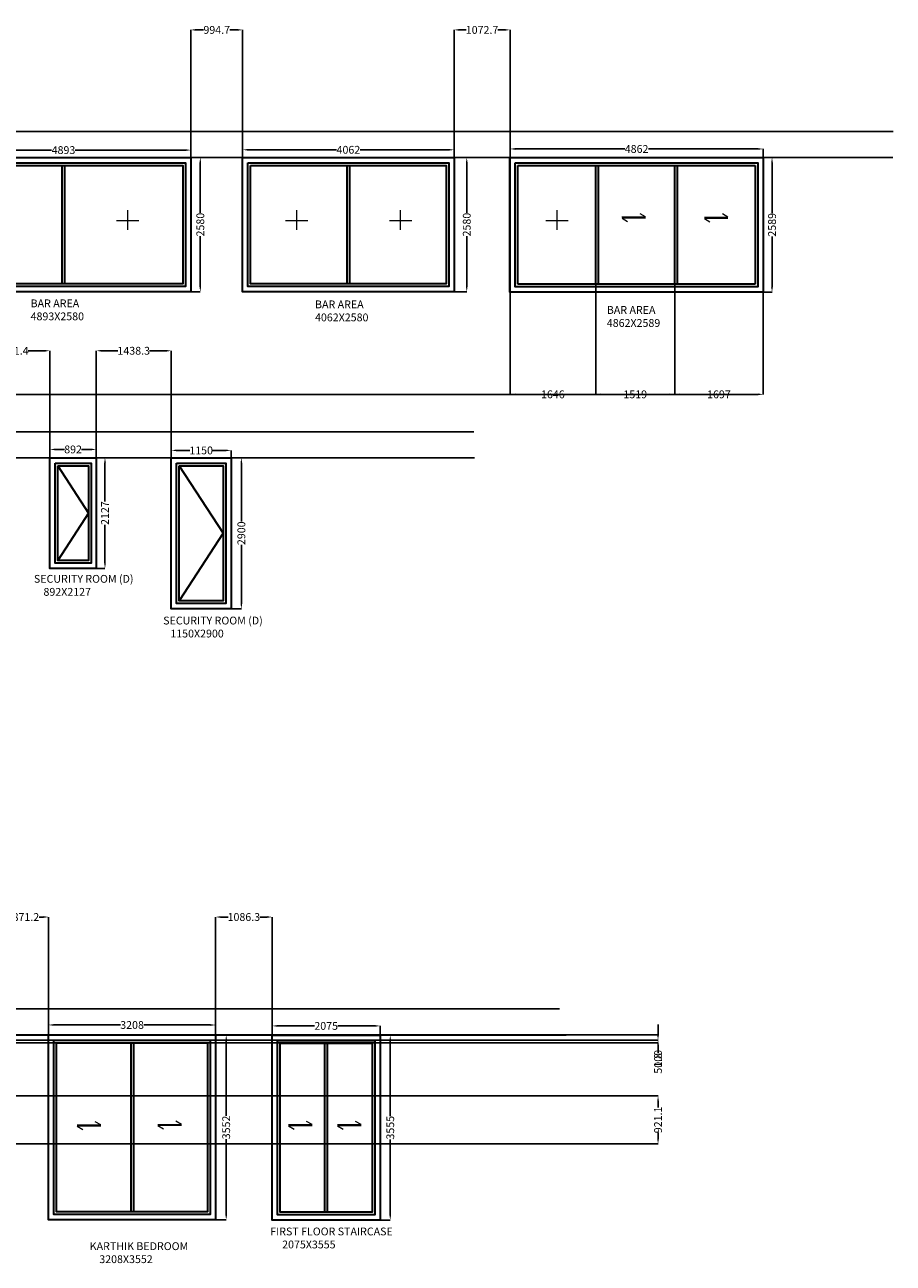
# Model space of a CAD drawing. Units: millimetres. Extents: x 16338 to 57165, y -4429 to 26237.
# Tile 6 of 6: x 40486 to 57165, y 2450 to 26237. Entities that reach past the tile are written whole.
import ezdxf

# ---------------------------------------------------------------- set-up
doc = ezdxf.new("R2010")
doc.units = ezdxf.units.MM
doc.header["$MEASUREMENT"] = 0
for name, color, linetype, lineweight in [('A-ANNO-DIMS', 5, 'Continuous', 18), ('A-ANNO-SYMB', 4, 'Continuous', 18), ('A-ANNO-TEXT', 3, 'Continuous', 18), ('A-ELEV', 8, 'Continuous', 25), ('A-GLAZ', 7, 'Continuous', 35)]:
    doc.layers.add(name, color=color, linetype=linetype, lineweight=lineweight)
doc.styles.get("Standard").update_dxf_attribs({"font": 'arial.ttf'})
doc.dimstyles.get("Standard").update_dxf_attribs({"dimtxt": 150, "dimasz": 100, "dimexe": 0.18, "dimexo": 0.0625, "dimgap": 0.09, "dimtad": 0, "dimdec": 0, "dimzin": 0, "dimdsep": 46, "dimtxsty": 'Standard', "dimcen": 0.09, "dimadec": 0, "dimazin": 0, "dimtfac": 1, "dimtdec": 0, "dimtofl": 0, "dimtmove": 0, "dimatfit": 3, "dimfxl": 1, "dimtolj": 1, "dimtzin": 0, "dimarcsym": 0})

# ---------------------------------------------------------------- blocks, each defined once
blk = doc.blocks.new('*D14')
at = {"layer": 'A-ANNO-DIMS', "color": 0, "lineweight": -2, "transparency": 16777216}
for p, q in [((38782, 23689), (38782, 23831)), ((38882, 23830), (41002, 23830)), ((43575, 23830), (41456, 23830)), ((43675, 23689), (43675, 23831))]:
    blk.add_line(p, q, dxfattribs=at)
at = {"layer": 'A-ANNO-DIMS', "color": 0, "transparency": 16777216}
for points in [[(38882, 23847), (38882, 23814), (38782, 23830)], [(43575, 23847), (43575, 23814), (43675, 23830)]]:
    blk.add_solid(points, dxfattribs=at)
at = {"layer": 'Defpoints', "color": 0, "transparency": 16777216}
for p in [(43675, 23830), (38782, 23689), (43675, 23689)]:
    blk.add_point(p, dxfattribs=at)
at = {"layer": 'A-ANNO-DIMS', "color": 0, "transparency": 16777216, "insert": (41229, 23830), "char_height": 150, "attachment_point": 5}
blk.add_mtext('\\A1;4893', dxfattribs=at)
blk = doc.blocks.new('*D15')
at = {"layer": 'A-ANNO-DIMS', "color": 0, "lineweight": -2, "transparency": 16777216}
for p, q in [((43675, 23689), (43857, 23689)), ((43857, 23589), (43857, 22624)), ((43857, 21209), (43857, 22174)), ((43675, 21109), (43857, 21109))]:
    blk.add_line(p, q, dxfattribs=at)
at = {"layer": 'A-ANNO-DIMS', "color": 0, "transparency": 16777216}
for points in [[(43840, 23589), (43873, 23589), (43857, 23689)], [(43840, 21209), (43873, 21209), (43857, 21109)]]:
    blk.add_solid(points, dxfattribs=at)
at = {"layer": 'Defpoints', "color": 0, "transparency": 16777216}
for p in [(43675, 23689), (43675, 21109), (43857, 21109)]:
    blk.add_point(p, dxfattribs=at)
at = {"layer": 'A-ANNO-DIMS', "color": 0, "transparency": 16777216, "insert": (43857, 22399), "char_height": 150, "attachment_point": 5, "rotation": 90}
blk.add_mtext('\\A1;2580', dxfattribs=at)
blk = doc.blocks.new('*D16')
at = {"layer": 'A-ANNO-DIMS', "color": 0, "lineweight": -2, "transparency": 16777216}
for p, q in [((44670, 23689), (44670, 23837)), ((44770, 23836), (46474, 23836)), ((48632, 23836), (46927, 23836)), ((48732, 23689), (48732, 23837))]:
    blk.add_line(p, q, dxfattribs=at)
at = {"layer": 'A-ANNO-DIMS', "color": 0, "transparency": 16777216}
for points in [[(44770, 23853), (44770, 23820), (44670, 23836)], [(48632, 23853), (48632, 23820), (48732, 23836)]]:
    blk.add_solid(points, dxfattribs=at)
at = {"layer": 'Defpoints', "color": 0, "transparency": 16777216}
for p in [(48732, 23836), (44670, 23689), (48732, 23689)]:
    blk.add_point(p, dxfattribs=at)
at = {"layer": 'A-ANNO-DIMS', "color": 0, "transparency": 16777216, "insert": (46701, 23836), "char_height": 150, "attachment_point": 5}
blk.add_mtext('\\A1;4062', dxfattribs=at)
blk = doc.blocks.new('*D17')
at = {"layer": 'A-ANNO-DIMS', "color": 0, "lineweight": -2, "transparency": 16777216}
for p, q in [((48732, 23689), (48974, 23689)), ((48974, 23589), (48974, 22624)), ((48974, 21209), (48974, 22174)), ((48732, 21109), (48974, 21109))]:
    blk.add_line(p, q, dxfattribs=at)
at = {"layer": 'A-ANNO-DIMS', "color": 0, "transparency": 16777216}
for points in [[(48957, 23589), (48990, 23589), (48974, 23689)], [(48957, 21209), (48990, 21209), (48974, 21109)]]:
    blk.add_solid(points, dxfattribs=at)
at = {"layer": 'Defpoints', "color": 0, "transparency": 16777216}
for p in [(48732, 23689), (48732, 21109), (48974, 21109)]:
    blk.add_point(p, dxfattribs=at)
at = {"layer": 'A-ANNO-DIMS', "color": 0, "transparency": 16777216, "insert": (48974, 22399), "char_height": 150, "attachment_point": 5, "rotation": 90}
blk.add_mtext('\\A1;2580', dxfattribs=at)
blk = doc.blocks.new('*D18')
at = {"layer": 'A-ANNO-DIMS', "color": 0, "lineweight": -2, "transparency": 16777216}
for p, q in [((49805, 23689), (49805, 23852)), ((49905, 23852), (52009, 23852)), ((54567, 23852), (52462, 23852)), ((54667, 23689), (54667, 23852))]:
    blk.add_line(p, q, dxfattribs=at)
at = {"layer": 'A-ANNO-DIMS', "color": 0, "transparency": 16777216}
for points in [[(49905, 23869), (49905, 23835), (49805, 23852)], [(54567, 23869), (54567, 23835), (54667, 23852)]]:
    blk.add_solid(points, dxfattribs=at)
at = {"layer": 'Defpoints', "color": 0, "transparency": 16777216}
for p in [(54667, 23852), (49805, 23689), (54667, 23689)]:
    blk.add_point(p, dxfattribs=at)
at = {"layer": 'A-ANNO-DIMS', "color": 0, "transparency": 16777216, "insert": (52236, 23852), "char_height": 150, "attachment_point": 5}
blk.add_mtext('\\A1;4862', dxfattribs=at)
blk = doc.blocks.new('*D19')
at = {"layer": 'A-ANNO-DIMS', "color": 0, "lineweight": -2, "transparency": 16777216}
for p, q in [((54667, 23689), (54837, 23689)), ((54837, 23589), (54837, 22620)), ((54837, 21200), (54837, 22169)), ((54667, 21100), (54837, 21100))]:
    blk.add_line(p, q, dxfattribs=at)
at = {"layer": 'A-ANNO-DIMS', "color": 0, "transparency": 16777216}
for points in [[(54820, 23589), (54854, 23589), (54837, 23689)], [(54820, 21200), (54854, 21200), (54837, 21100)]]:
    blk.add_solid(points, dxfattribs=at)
at = {"layer": 'Defpoints', "color": 0, "transparency": 16777216}
for p in [(54667, 23689), (54667, 21100), (54837, 21100)]:
    blk.add_point(p, dxfattribs=at)
at = {"layer": 'A-ANNO-DIMS', "color": 0, "transparency": 16777216, "insert": (54837, 22395), "char_height": 150, "attachment_point": 5, "rotation": 90}
blk.add_mtext('\\A1;2589', dxfattribs=at)
blk = doc.blocks.new('*D36')
at = {"layer": 'A-ANNO-DIMS', "color": 0, "lineweight": -2, "transparency": 16777216}
for p, q in [((40967, 17921), (40967, 18081)), ((41067, 18081), (41248, 18081)), ((41759, 18081), (41578, 18081)), ((41859, 17921), (41859, 18081))]:
    blk.add_line(p, q, dxfattribs=at)
at = {"layer": 'A-ANNO-DIMS', "color": 0, "transparency": 16777216}
for points in [[(41067, 18097), (41067, 18064), (40967, 18081)], [(41759, 18097), (41759, 18064), (41859, 18081)]]:
    blk.add_solid(points, dxfattribs=at)
at = {"layer": 'Defpoints', "color": 0, "transparency": 16777216}
for p in [(41859, 18081), (40967, 17921), (41859, 17921)]:
    blk.add_point(p, dxfattribs=at)
at = {"layer": 'A-ANNO-DIMS', "color": 0, "transparency": 16777216, "insert": (41413, 18081), "char_height": 150, "attachment_point": 5}
blk.add_mtext('\\A1;892', dxfattribs=at)
blk = doc.blocks.new('*D37')
at = {"layer": 'A-ANNO-DIMS', "color": 0, "lineweight": -2, "transparency": 16777216}
for p, q in [((41859, 17921), (42026, 17921)), ((42026, 17821), (42026, 17083)), ((42026, 15894), (42026, 16632)), ((41859, 15794), (42026, 15794))]:
    blk.add_line(p, q, dxfattribs=at)
at = {"layer": 'A-ANNO-DIMS', "color": 0, "transparency": 16777216}
for points in [[(42010, 17821), (42043, 17821), (42026, 17921)], [(42010, 15894), (42043, 15894), (42026, 15794)]]:
    blk.add_solid(points, dxfattribs=at)
at = {"layer": 'Defpoints', "color": 0, "transparency": 16777216}
for p in [(41859, 17921), (41859, 15794), (42026, 15794)]:
    blk.add_point(p, dxfattribs=at)
at = {"layer": 'A-ANNO-DIMS', "color": 0, "transparency": 16777216, "insert": (42026, 16858), "char_height": 150, "attachment_point": 5, "rotation": 90}
blk.add_mtext('\\A1;2127', dxfattribs=at)
blk = doc.blocks.new('*D38')
at = {"layer": 'A-ANNO-DIMS', "color": 0, "lineweight": -2, "transparency": 16777216}
for p, q in [((43298, 17921), (43298, 18062)), ((43398, 18062), (43656, 18062)), ((44348, 18062), (44089, 18062)), ((44448, 17921), (44448, 18062))]:
    blk.add_line(p, q, dxfattribs=at)
at = {"layer": 'A-ANNO-DIMS', "color": 0, "transparency": 16777216}
for points in [[(43398, 18079), (43398, 18046), (43298, 18062)], [(44348, 18079), (44348, 18046), (44448, 18062)]]:
    blk.add_solid(points, dxfattribs=at)
at = {"layer": 'Defpoints', "color": 0, "transparency": 16777216}
for p in [(43298, 17921), (44448, 18062), (44448, 17921)]:
    blk.add_point(p, dxfattribs=at)
at = {"layer": 'A-ANNO-DIMS', "color": 0, "transparency": 16777216, "insert": (43873, 18062), "char_height": 150, "attachment_point": 5}
blk.add_mtext('\\A1;1150', dxfattribs=at)
blk = doc.blocks.new('*D39')
at = {"layer": 'A-ANNO-DIMS', "color": 0, "lineweight": -2, "transparency": 16777216}
for p, q in [((44448, 17921), (44646, 17921)), ((44645, 17821), (44645, 16696)), ((44645, 15121), (44645, 16246)), ((44448, 15021), (44646, 15021))]:
    blk.add_line(p, q, dxfattribs=at)
at = {"layer": 'A-ANNO-DIMS', "color": 0, "transparency": 16777216}
for points in [[(44629, 17821), (44662, 17821), (44645, 17921)], [(44629, 15121), (44662, 15121), (44645, 15021)]]:
    blk.add_solid(points, dxfattribs=at)
at = {"layer": 'Defpoints', "color": 0, "transparency": 16777216}
for p in [(44448, 17921), (44448, 15021), (44645, 15021)]:
    blk.add_point(p, dxfattribs=at)
at = {"layer": 'A-ANNO-DIMS', "color": 0, "transparency": 16777216, "insert": (44645, 16471), "char_height": 150, "attachment_point": 5, "rotation": 90}
blk.add_mtext('\\A1;2900', dxfattribs=at)
blk = doc.blocks.new('*D67')
at = {"layer": 'A-ANNO-DIMS', "color": 0, "lineweight": -2, "transparency": 16777216}
for p, q in [((40942, 6834), (40942, 7026)), ((41042, 7026), (42322, 7026)), ((44050, 7026), (42770, 7026)), ((44150, 6834), (44150, 7026))]:
    blk.add_line(p, q, dxfattribs=at)
at = {"layer": 'A-ANNO-DIMS', "color": 0, "transparency": 16777216}
for points in [[(41042, 7043), (41042, 7009), (40942, 7026)], [(44050, 7043), (44050, 7009), (44150, 7026)]]:
    blk.add_solid(points, dxfattribs=at)
at = {"layer": 'Defpoints', "color": 0, "transparency": 16777216}
for p in [(44150, 7026), (40942, 6834), (44150, 6834)]:
    blk.add_point(p, dxfattribs=at)
at = {"layer": 'A-ANNO-DIMS', "color": 0, "transparency": 16777216, "insert": (42546, 7026), "char_height": 150, "attachment_point": 5}
blk.add_mtext('\\A1;3208', dxfattribs=at)
blk = doc.blocks.new('*D68')
at = {"layer": 'A-ANNO-DIMS', "color": 0, "lineweight": -2, "transparency": 16777216}
for p, q in [((44150, 6834), (44355, 6834)), ((44354, 6734), (44354, 5281)), ((44354, 3382), (44354, 4835)), ((44150, 3282), (44355, 3282))]:
    blk.add_line(p, q, dxfattribs=at)
at = {"layer": 'A-ANNO-DIMS', "color": 0, "transparency": 16777216}
for points in [[(44338, 6734), (44371, 6734), (44354, 6834)], [(44338, 3382), (44371, 3382), (44354, 3282)]]:
    blk.add_solid(points, dxfattribs=at)
at = {"layer": 'Defpoints', "color": 0, "transparency": 16777216}
for p in [(44150, 6834), (44150, 3282), (44354, 3282)]:
    blk.add_point(p, dxfattribs=at)
at = {"layer": 'A-ANNO-DIMS', "color": 0, "transparency": 16777216, "insert": (44354, 5058), "char_height": 150, "attachment_point": 5, "rotation": 90}
blk.add_mtext('\\A1;3552', dxfattribs=at)
blk = doc.blocks.new('*D69')
at = {"layer": 'A-ANNO-DIMS', "color": 0, "lineweight": -2, "transparency": 16777216}
for p, q in [((45236, 6830), (45236, 7008)), ((45336, 7008), (46048, 7008)), ((47211, 7008), (46500, 7008)), ((47311, 6830), (47311, 7008))]:
    blk.add_line(p, q, dxfattribs=at)
at = {"layer": 'A-ANNO-DIMS', "color": 0, "transparency": 16777216}
for points in [[(45336, 7025), (45336, 6992), (45236, 7008)], [(47211, 7025), (47211, 6992), (47311, 7008)]]:
    blk.add_solid(points, dxfattribs=at)
at = {"layer": 'Defpoints', "color": 0, "transparency": 16777216}
for p in [(47311, 7008), (45236, 6830), (47311, 6830)]:
    blk.add_point(p, dxfattribs=at)
at = {"layer": 'A-ANNO-DIMS', "color": 0, "transparency": 16777216, "insert": (46274, 7008), "char_height": 150, "attachment_point": 5}
blk.add_mtext('\\A1;2075', dxfattribs=at)
blk = doc.blocks.new('*D70')
at = {"layer": 'A-ANNO-DIMS', "color": 0, "lineweight": -2, "transparency": 16777216}
for p, q in [((47311, 6830), (47505, 6830)), ((47505, 6730), (47505, 5277)), ((47505, 3375), (47505, 4828)), ((47311, 3275), (47505, 3275))]:
    blk.add_line(p, q, dxfattribs=at)
at = {"layer": 'A-ANNO-DIMS', "color": 0, "transparency": 16777216}
for points in [[(47488, 6730), (47521, 6730), (47505, 6830)], [(47488, 3375), (47521, 3375), (47505, 3275)]]:
    blk.add_solid(points, dxfattribs=at)
at = {"layer": 'Defpoints', "color": 0, "transparency": 16777216}
for p in [(47311, 6830), (47311, 3275), (47505, 3275)]:
    blk.add_point(p, dxfattribs=at)
at = {"layer": 'A-ANNO-DIMS', "color": 0, "transparency": 16777216, "insert": (47505, 5053), "char_height": 150, "attachment_point": 5, "rotation": 90}
blk.add_mtext('\\A1;3555', dxfattribs=at)
blk = doc.blocks.new('SLIDE-ARROW-L')
for p, q in [((454, 0), (347, 62)), ((0, 0), (454, 0))]:
    blk.add_line(p, q)
blk = doc.blocks.new('*D89')
at = {"layer": 'A-ANNO-DIMS', "color": 0, "lineweight": -2, "transparency": 16777216}
for p, q in [((43675, 23689), (43675, 26139)), ((43775, 26139), (43919, 26139)), ((44570, 26139), (44426, 26139)), ((44670, 23689), (44670, 26139))]:
    blk.add_line(p, q, dxfattribs=at)
at = {"layer": 'A-ANNO-DIMS', "color": 0, "transparency": 16777216}
for points in [[(43775, 26156), (43775, 26122), (43675, 26139)], [(44570, 26156), (44570, 26122), (44670, 26139)]]:
    blk.add_solid(points, dxfattribs=at)
at = {"layer": 'Defpoints', "color": 0, "transparency": 16777216}
for p in [(44670, 26139), (43675, 23689), (44670, 23689)]:
    blk.add_point(p, dxfattribs=at)
at = {"layer": 'A-ANNO-DIMS', "color": 0, "transparency": 16777216, "insert": (44172, 26139), "char_height": 150, "attachment_point": 5}
blk.add_mtext('\\A1;994.7', dxfattribs=at)
blk = doc.blocks.new('*D90')
at = {"layer": 'A-ANNO-DIMS', "color": 0, "lineweight": -2, "transparency": 16777216}
for p, q in [((48732, 23689), (48732, 26139)), ((48832, 26139), (48964, 26139)), ((49705, 26139), (49573, 26139)), ((49805, 23689), (49805, 26139))]:
    blk.add_line(p, q, dxfattribs=at)
at = {"layer": 'A-ANNO-DIMS', "color": 0, "transparency": 16777216}
for points in [[(48832, 26156), (48832, 26122), (48732, 26139)], [(49705, 26156), (49705, 26122), (49805, 26139)]]:
    blk.add_solid(points, dxfattribs=at)
at = {"layer": 'Defpoints', "color": 0, "transparency": 16777216}
for p in [(49805, 26139), (48732, 23689), (49805, 23689)]:
    blk.add_point(p, dxfattribs=at)
at = {"layer": 'A-ANNO-DIMS', "color": 0, "transparency": 16777216, "insert": (49268, 26139), "char_height": 150, "attachment_point": 5}
blk.add_mtext('\\A1;1072.7', dxfattribs=at)
blk = doc.blocks.new('*D91')
at = {"layer": 'A-ANNO-DIMS', "color": 0, "lineweight": -2, "transparency": 16777216}
for p, q in [((19179, 21089), (19179, 19139)), ((54667, 21100), (54667, 19139)), ((19279, 19139), (36641, 19139)), ((54567, 19139), (37205, 19139))]:
    blk.add_line(p, q, dxfattribs=at)
at = {"layer": 'A-ANNO-DIMS', "color": 0, "transparency": 16777216}
for points in [[(19279, 19156), (19279, 19122), (19179, 19139)], [(54567, 19156), (54567, 19122), (54667, 19139)]]:
    blk.add_solid(points, dxfattribs=at)
at = {"layer": 'Defpoints', "color": 0, "transparency": 16777216}
for p in [(19179, 21089), (54667, 21100), (54667, 19139)]:
    blk.add_point(p, dxfattribs=at)
at = {"layer": 'A-ANNO-DIMS', "color": 0, "transparency": 16777216, "insert": (36923, 19139), "char_height": 150, "attachment_point": 5}
blk.add_mtext('\\A1;35487', dxfattribs=at)
blk = doc.blocks.new('*D92')
at = {"layer": 'A-ANNO-DIMS', "color": 0, "lineweight": -2, "transparency": 16777216}
for p, q in [((49805, 23689), (49805, 19139)), ((51451, 23537), (51451, 19139)), ((49905, 19139), (50411, 19139)), ((51351, 19139), (50845, 19139))]:
    blk.add_line(p, q, dxfattribs=at)
at = {"layer": 'A-ANNO-DIMS', "color": 0, "transparency": 16777216}
for points in [[(49905, 19156), (49905, 19122), (49805, 19139)], [(51351, 19156), (51351, 19122), (51451, 19139)]]:
    blk.add_solid(points, dxfattribs=at)
at = {"layer": 'Defpoints', "color": 0, "transparency": 16777216}
for p in [(49805, 23689), (51451, 23537), (51451, 19139)]:
    blk.add_point(p, dxfattribs=at)
at = {"layer": 'A-ANNO-DIMS', "color": 0, "transparency": 16777216, "insert": (50628, 19139), "char_height": 150, "attachment_point": 5}
blk.add_mtext('\\A1;1646', dxfattribs=at)
blk = doc.blocks.new('*D93')
at = {"layer": 'A-ANNO-DIMS', "color": 0, "lineweight": -2, "transparency": 16777216}
for p, q in [((51451, 23537), (51451, 19139)), ((52970, 23537), (52970, 19139)), ((51551, 19139), (51993, 19139)), ((52870, 19139), (52427, 19139))]:
    blk.add_line(p, q, dxfattribs=at)
at = {"layer": 'A-ANNO-DIMS', "color": 0, "transparency": 16777216}
for points in [[(51551, 19156), (51551, 19122), (51451, 19139)], [(52870, 19156), (52870, 19122), (52970, 19139)]]:
    blk.add_solid(points, dxfattribs=at)
at = {"layer": 'Defpoints', "color": 0, "transparency": 16777216}
for p in [(51451, 23537), (52970, 23537), (52970, 19139)]:
    blk.add_point(p, dxfattribs=at)
at = {"layer": 'A-ANNO-DIMS', "color": 0, "transparency": 16777216, "insert": (52210, 19139), "char_height": 150, "attachment_point": 5}
blk.add_mtext('\\A1;1519', dxfattribs=at)
blk = doc.blocks.new('*D94')
at = {"layer": 'A-ANNO-DIMS', "color": 0, "lineweight": -2, "transparency": 16777216}
for p, q in [((54667, 23689), (54667, 19139)), ((52970, 23537), (52970, 19139)), ((53070, 19139), (53601, 19139)), ((54567, 19139), (54035, 19139))]:
    blk.add_line(p, q, dxfattribs=at)
at = {"layer": 'A-ANNO-DIMS', "color": 0, "transparency": 16777216}
for points in [[(53070, 19156), (53070, 19122), (52970, 19139)], [(54567, 19156), (54567, 19122), (54667, 19139)]]:
    blk.add_solid(points, dxfattribs=at)
at = {"layer": 'Defpoints', "color": 0, "transparency": 16777216}
for p in [(54667, 23689), (52970, 23537), (54667, 19139)]:
    blk.add_point(p, dxfattribs=at)
at = {"layer": 'A-ANNO-DIMS', "color": 0, "transparency": 16777216, "insert": (53818, 19139), "char_height": 150, "attachment_point": 5}
blk.add_mtext('\\A1;1697', dxfattribs=at)
blk = doc.blocks.new('*D102')
at = {"layer": 'A-ANNO-DIMS', "color": 0, "lineweight": -2, "transparency": 16777216}
for p, q in [((39526, 17921), (39526, 19976)), ((39626, 19976), (39943, 19976)), ((40867, 19976), (40551, 19976)), ((40967, 17921), (40967, 19976))]:
    blk.add_line(p, q, dxfattribs=at)
at = {"layer": 'A-ANNO-DIMS', "color": 0, "transparency": 16777216}
for points in [[(39626, 19993), (39626, 19959), (39526, 19976)], [(40867, 19993), (40867, 19959), (40967, 19976)]]:
    blk.add_solid(points, dxfattribs=at)
at = {"layer": 'Defpoints', "color": 0, "transparency": 16777216}
for p in [(40967, 19976), (39526, 17921), (40967, 17921)]:
    blk.add_point(p, dxfattribs=at)
at = {"layer": 'A-ANNO-DIMS', "color": 0, "transparency": 16777216, "insert": (40247, 19976), "char_height": 150, "attachment_point": 5}
blk.add_mtext('\\A1;1441.4', dxfattribs=at)
blk = doc.blocks.new('*D103')
at = {"layer": 'A-ANNO-DIMS', "color": 0, "lineweight": -2, "transparency": 16777216}
for p, q in [((41859, 17921), (41859, 19976)), ((41959, 19976), (42274, 19976)), ((43198, 19976), (42883, 19976)), ((43298, 17921), (43298, 19976))]:
    blk.add_line(p, q, dxfattribs=at)
at = {"layer": 'A-ANNO-DIMS', "color": 0, "transparency": 16777216}
for points in [[(41959, 19993), (41959, 19959), (41859, 19976)], [(43198, 19993), (43198, 19959), (43298, 19976)]]:
    blk.add_solid(points, dxfattribs=at)
at = {"layer": 'Defpoints', "color": 0, "transparency": 16777216}
for p in [(43298, 19976), (41859, 17921), (43298, 17921)]:
    blk.add_point(p, dxfattribs=at)
at = {"layer": 'A-ANNO-DIMS', "color": 0, "transparency": 16777216, "insert": (42578, 19976), "char_height": 150, "attachment_point": 5}
blk.add_mtext('\\A1;1438.3', dxfattribs=at)
blk = doc.blocks.new('*D116')
at = {"layer": 'A-ANNO-DIMS', "color": 0, "lineweight": -2, "transparency": 16777216}
for p, q in [((40071, 6835), (40071, 9100)), ((40171, 9100), (40254, 9100)), ((40842, 9100), (40759, 9100)), ((40942, 6834), (40942, 9100))]:
    blk.add_line(p, q, dxfattribs=at)
at = {"layer": 'A-ANNO-DIMS', "color": 0, "transparency": 16777216}
for points in [[(40171, 9117), (40171, 9083), (40071, 9100)], [(40842, 9117), (40842, 9083), (40942, 9100)]]:
    blk.add_solid(points, dxfattribs=at)
at = {"layer": 'Defpoints', "color": 0, "transparency": 16777216}
for p in [(40942, 9100), (40071, 6835), (40942, 6834)]:
    blk.add_point(p, dxfattribs=at)
at = {"layer": 'A-ANNO-DIMS', "color": 0, "transparency": 16777216, "insert": (40507, 9100), "char_height": 150, "attachment_point": 5}
blk.add_mtext('\\A1;871.2', dxfattribs=at)
blk = doc.blocks.new('*D117')
at = {"layer": 'A-ANNO-DIMS', "color": 0, "lineweight": -2, "transparency": 16777216}
for p, q in [((44150, 6834), (44150, 9100)), ((44250, 9100), (44389, 9100)), ((45136, 9100), (44998, 9100)), ((45236, 6830), (45236, 9100))]:
    blk.add_line(p, q, dxfattribs=at)
at = {"layer": 'A-ANNO-DIMS', "color": 0, "transparency": 16777216}
for points in [[(44250, 9117), (44250, 9083), (44150, 9100)], [(45136, 9117), (45136, 9083), (45236, 9100)]]:
    blk.add_solid(points, dxfattribs=at)
at = {"layer": 'Defpoints', "color": 0, "transparency": 16777216}
for p in [(45236, 9100), (44150, 6834), (45236, 6830)]:
    blk.add_point(p, dxfattribs=at)
at = {"layer": 'A-ANNO-DIMS', "color": 0, "transparency": 16777216, "insert": (44693, 9100), "char_height": 150, "attachment_point": 5}
blk.add_mtext('\\A1;1086.3', dxfattribs=at)
blk = doc.blocks.new('*D126')
at = {"layer": 'A-ANNO-DIMS', "color": 0, "lineweight": -2, "transparency": 16777216}
for p, q in [((52648, 6935), (52648, 7035)), ((23725, 6735), (52648, 6735)), ((23825, 6835), (52648, 6835)), ((52648, 6635), (52648, 6535))]:
    blk.add_line(p, q, dxfattribs=at)
at = {"layer": 'A-ANNO-DIMS', "color": 0, "transparency": 16777216}
for points in [[(52631, 6935), (52665, 6935), (52648, 6835)], [(52631, 6635), (52665, 6635), (52648, 6735)]]:
    blk.add_solid(points, dxfattribs=at)
at = {"layer": 'Defpoints', "color": 0, "transparency": 16777216}
for p in [(23725, 6735), (23825, 6835), (52648, 6735)]:
    blk.add_point(p, dxfattribs=at)
at = {"layer": 'A-ANNO-DIMS', "color": 0, "transparency": 16777216, "insert": (52648, 6377), "char_height": 150, "attachment_point": 5, "rotation": 90}
blk.add_mtext('\\A1;100', dxfattribs=at)
blk = doc.blocks.new('*D127')
at = {"layer": 'A-ANNO-DIMS', "color": 0, "lineweight": -2, "transparency": 16777216}
for p, q in [((52648, 6835), (52648, 6935)), ((23674, 6684), (52648, 6684)), ((23725, 6735), (52648, 6735)), ((52648, 6584), (52648, 6484))]:
    blk.add_line(p, q, dxfattribs=at)
at = {"layer": 'A-ANNO-DIMS', "color": 0, "transparency": 16777216}
for points in [[(52631, 6835), (52665, 6835), (52648, 6735)], [(52631, 6584), (52665, 6584), (52648, 6684)]]:
    blk.add_solid(points, dxfattribs=at)
at = {"layer": 'Defpoints', "color": 0, "transparency": 16777216}
for p in [(23674, 6684), (23725, 6735), (52648, 6684)]:
    blk.add_point(p, dxfattribs=at)
at = {"layer": 'A-ANNO-DIMS', "color": 0, "transparency": 16777216, "insert": (52648, 6289), "char_height": 150, "attachment_point": 5, "rotation": 90}
blk.add_mtext('\\A1;50.8', dxfattribs=at)
blk = doc.blocks.new('*D132')
at = {"layer": 'A-ANNO-DIMS', "color": 0, "lineweight": -2, "transparency": 16777216}
for p, q in [((23674, 5663), (52648, 5663)), ((52648, 5563), (52648, 5441)), ((52648, 4842), (52648, 4964)), ((23616, 4742), (52648, 4742))]:
    blk.add_line(p, q, dxfattribs=at)
at = {"layer": 'A-ANNO-DIMS', "color": 0, "transparency": 16777216}
for points in [[(52631, 5563), (52665, 5563), (52648, 5663)], [(52631, 4842), (52665, 4842), (52648, 4742)]]:
    blk.add_solid(points, dxfattribs=at)
at = {"layer": 'Defpoints', "color": 0, "transparency": 16777216}
for p in [(23674, 5663), (52648, 5663), (23616, 4742)]:
    blk.add_point(p, dxfattribs=at)
at = {"layer": 'A-ANNO-DIMS', "color": 0, "transparency": 16777216, "insert": (52648, 5203), "char_height": 150, "attachment_point": 5, "rotation": 90}
blk.add_mtext('\\A1;921.1', dxfattribs=at)

msp = doc.modelspace()

# ---------------------------------------------------------------- linework, layer by layer
at = {"layer": 'A-ANNO-DIMS'}
for p in [(51475.99, 21252.42), (52995.06, 21252.42)]:
    msp.add_point(p, dxfattribs=at)
at = {"layer": 'A-ANNO-SYMB'}
for p, q in [((42462.86, 22298.38), (42462.86, 22676.6)), ((45709.68, 22298.38), (45709.68, 22676.6)), ((47702.87, 22298.38), (47702.87, 22676.6)), ((50708.19, 22298.38), (50708.19, 22676.6)), ((42248.45, 22479.47), (42677.27, 22479.47)), ((45495.27, 22479.47), (45924.09, 22479.47)), ((47488.46, 22479.47), (47917.28, 22479.47)), ((50493.78, 22479.47), (50922.6, 22479.47))]:
    msp.add_line(p, q, dxfattribs=at)
at = {"layer": 'A-ELEV'}
for p, q in [((18334.8, 24189.02), (57164.77, 24189.02)), ((18334.8, 23689.02), (57154.46, 23689.02)), ((18334.8, 18421.15), (49111.23, 18421.15)), ((18334.8, 17921.15), (49122.07, 17921.15)), ((18209.23, 7335.1), (50757.08, 7335.1)), ((18201.83, 6834.85), (50882.91, 6829.39))]:
    msp.add_line(p, q, dxfattribs=at)
at = {"layer": 'A-GLAZ'}
for p, q in [((41203.19, 21261.42), (41203.19, 23536.62)), ((41253.99, 21261.42), (41253.99, 23536.62)), ((46675.42, 21261.42), (46675.42, 23536.62)), ((46726.22, 21261.42), (46726.22, 23536.62)), ((49956.93, 23536.62), (54514.13, 23536.62)), ((49956.93, 21252.42), (49956.93, 23536.62)), ((51450.59, 21252.42), (51450.59, 23536.62)), ((51501.39, 21252.42), (51501.39, 23536.62)), ((52969.66, 21252.42), (52969.66, 23536.62)), ((53020.46, 21252.42), (53020.46, 23536.62)), ((54514.13, 23536.62), (54514.13, 21252.42)), ((54514.13, 21252.42), (49956.93, 21252.42)), ((41119.74, 17768.75), (41706.94, 16857.65)), ((43450.06, 17768.75), (44295.26, 16471.15)), ((41706.94, 16857.65), (41119.74, 15946.55)), ((44295.26, 16471.15), (43450.06, 15173.55)), ((42520.74, 6681.8), (42520.74, 3434.6)), ((42571.54, 6681.8), (42571.54, 3434.6)), ((46248.52, 3427.73), (46248.52, 6677.93)), ((46299.32, 3427.73), (46299.32, 6677.93))]:
    msp.add_line(p, q, dxfattribs=at)
for points in [[(38782.09, 23689.02), (43675.09, 23689.02), (43675.09, 21109.02), (38782.09, 21109.02)], [(38883.69, 23587.42), (43573.49, 23587.42), (43573.49, 21210.62), (38883.69, 21210.62)], [(44669.82, 23689.02), (48731.82, 23689.02), (48731.82, 21109.02), (44669.82, 21109.02)], [(44771.42, 23587.42), (48630.22, 23587.42), (48630.22, 21210.62), (44771.42, 21210.62)], [(49804.53, 23689.02), (54666.53, 23689.02), (54666.53, 21100.02), (49804.53, 21100.02)], [(49906.13, 23587.42), (54564.93, 23587.42), (54564.93, 21201.62), (49906.13, 21201.62)], [(38934.49, 23536.62), (43522.69, 23536.62), (43522.69, 21261.42), (38934.49, 21261.42)], [(44822.22, 23536.62), (48579.42, 23536.62), (48579.42, 21261.42), (44822.22, 21261.42)], [(40967.34, 17921.15), (41859.34, 17921.15), (41859.34, 15794.15), (40967.34, 15794.15)], [(43297.66, 17921.15), (44447.66, 17921.15), (44447.66, 15021.15), (43297.66, 15021.15)], [(41068.94, 17819.55), (41757.74, 17819.55), (41757.74, 15895.75), (41068.94, 15895.75)], [(41119.74, 17768.75), (41706.94, 17768.75), (41706.94, 15946.55), (41119.74, 15946.55)], [(43399.26, 17819.55), (44346.06, 17819.55), (44346.06, 15122.75), (43399.26, 15122.75)], [(43450.06, 17768.75), (44295.26, 17768.75), (44295.26, 15173.55), (43450.06, 15173.55)], [(40942.14, 6834.2), (44150.14, 6834.2), (44150.14, 3282.2), (40942.14, 3282.2)], [(41043.74, 6732.6), (44048.54, 6732.6), (44048.54, 3383.8), (41043.74, 3383.8)], [(41094.54, 6681.8), (43997.74, 6681.8), (43997.74, 3434.6), (41094.54, 3434.6)], [(45236.42, 6830.33), (47311.42, 6830.33), (47311.42, 3275.33), (45236.42, 3275.33)], [(45338.02, 6728.73), (47209.82, 6728.73), (47209.82, 3376.93), (45338.02, 3376.93)], [(45388.82, 6677.93), (47159.02, 6677.93), (47159.02, 3427.73), (45388.82, 3427.73)]]:
    msp.add_lwpolyline(points, close=True, dxfattribs=at)

# ---------------------------------------------------------------- block references
at = {"layer": 'A-ANNO-SYMB'}
for p in [(51955.59, 22545.86), (53537.03, 22541.17), (41490.33, 5106.84), (43041.75, 5117.24), (45552.37, 5113.38), (46491.06, 5113.38)]:
    msp.add_blockref('SLIDE-ARROW-L', p, dxfattribs=at)
at = {"layer": 'A-ANNO-SYMB', "rotation": 180}
for p in [(52409.79, 22521.2), (53991.23, 22516.52), (41944.53, 5082.19), (43495.95, 5092.59), (46006.57, 5088.72), (46945.26, 5088.72)]:
    msp.add_blockref('SLIDE-ARROW-L', p, dxfattribs=at)

# ---------------------------------------------------------------- texts
at = {"layer": 'A-ANNO-TEXT', "char_height": 150, "attachment_point": 1}
for s, insert in [('BAR AREA\\P4893X2580', (40597.6, 20961.52)), ('BAR AREA\\P4062X2580', (46060.13, 20941.98)), ('BAR AREA\\P4862X2589', (51664.52, 20834.71)), ('SECURITY ROOM (D)\\P    892X2127', (40661.38, 15670.31)), ('SECURITY ROOM (D)\\P   1150X2900', (43143.97, 14869.2)), ('FIRST FLOOR STAIRCASE\\P     2075X3555', (45199.59, 3135.03)), ('\\PKARTHIK BEDROOM\\P    3208X3552', (41733.24, 3102.75))]:
    msp.add_mtext_dynamic_manual_height_columns(s, width=7094.9176, gutter_width=1, heights=[0], dxfattribs=dict(at, insert=insert))

# ---------------------------------------------------------------- dimensions: what is measured, and where the dimension line sits
at = {"layer": 'A-ANNO-DIMS'}
for base, p1, p2, override, picture, middle in [((44669.82, 26139.02), (43675.09, 23689.02), (44669.82, 23689.02), {"dimdec": 1, "dimlfac": 1, "dimrnd": 0, "dimzin": 0, "dimdsep": 46, "dimlunit": 2}, '*D89', (44172.45, 26139.02)), ((49804.53, 26139.02), (48731.82, 23689.02), (49804.53, 23689.02), {"dimdec": 1, "dimlfac": 1, "dimrnd": 0, "dimzin": 0, "dimdsep": 46, "dimlunit": 2}, '*D90', (49268.17, 26139.02)), ((43675.09, 23830.45), (38782.09, 23689.02), (43675.09, 23689.02), {"dimclrd": 0, "dimclre": 0, "dimclrt": 0}, '*D14', (41228.59, 23830.45)), ((48731.82, 23836.37), (44669.82, 23689.02), (48731.82, 23689.02), {"dimclrd": 0, "dimclre": 0, "dimclrt": 0}, '*D16', (46700.82, 23836.37)), ((54666.53, 23851.85), (49804.53, 23689.02), (54666.53, 23689.02), {"dimclrd": 0, "dimclre": 0, "dimclrt": 0}, '*D18', (52235.53, 23851.85)), ((51450.59, 19139.02), (49804.53, 23689.02), (51450.59, 23536.62), {"dimdec": 0, "dimlfac": 1, "dimrnd": 0, "dimzin": 0, "dimdsep": 46, "dimlunit": 2}, '*D92', (50627.56, 19139.02)), ((54666.53, 19139.02), (52969.66, 23536.62), (54666.53, 23689.02), {"dimdec": 0, "dimlfac": 1, "dimrnd": 0, "dimzin": 0, "dimdsep": 46, "dimlunit": 2}, '*D94', (53818.09, 19139.02)), ((52969.66, 19139.02), (51450.59, 23536.62), (52969.66, 23536.62), {"dimdec": 0, "dimlfac": 1, "dimrnd": 0, "dimzin": 0, "dimdsep": 46, "dimlunit": 2}, '*D93', (52210.13, 19139.02)), ((54666.53, 19139.02), (19179.17, 21089.02), (54666.53, 21100.02), {"dimdec": 0, "dimlfac": 1, "dimrnd": 0, "dimzin": 0, "dimdsep": 46, "dimlunit": 2}, '*D91', (36922.85, 19139.02)), ((40967.34, 19976.15), (39525.93, 17921.15), (40967.34, 17921.15), {"dimdec": 1, "dimlfac": 1, "dimrnd": 0, "dimzin": 0, "dimdsep": 46, "dimlunit": 2}, '*D102', (40246.63, 19976.15)), ((43297.66, 19976.15), (41859.34, 17921.15), (43297.66, 17921.15), {"dimdec": 1, "dimlfac": 1, "dimrnd": 0, "dimzin": 0, "dimdsep": 46, "dimlunit": 2}, '*D103', (42578.5, 19976.15)), ((41859.34, 18080.51), (40967.34, 17921.15), (41859.34, 17921.15), {"dimclrd": 0, "dimclre": 0, "dimclrt": 0}, '*D36', (41413.34, 18080.51)), ((44447.66, 18062.23), (43297.66, 17921.15), (44447.66, 17921.15), {"dimclrd": 0, "dimclre": 0, "dimclrt": 0}, '*D38', (43872.66, 18062.23)), ((40942.14, 9100.1), (40070.97, 6835.1), (40942.14, 6834.2), {"dimdec": 1, "dimlfac": 1, "dimrnd": 0, "dimzin": 0, "dimdsep": 46, "dimlunit": 2}, '*D116', (40506.55, 9100.1)), ((45236.42, 9100.1), (44150.14, 6834.2), (45236.42, 6830.33), {"dimdec": 1, "dimlfac": 1, "dimrnd": 0, "dimzin": 0, "dimdsep": 46, "dimlunit": 2}, '*D117', (44693.28, 9100.1)), ((44150.14, 7025.88), (40942.14, 6834.2), (44150.14, 6834.2), {"dimclrd": 0, "dimclre": 0, "dimclrt": 0}, '*D67', (42546.14, 7025.88)), ((47311.42, 7008.29), (45236.42, 6830.33), (47311.42, 6830.33), {"dimclrd": 0, "dimclre": 0, "dimclrt": 0}, '*D69', (46273.92, 7008.29))]:
    dim = msp.add_linear_dim(base=base, p1=p1, p2=p2, dimstyle='Standard', override=override, dxfattribs=at)
    dim.commit()
    dim.dimension.update_dxf_attribs({"geometry": picture, "text_midpoint": middle})
for base, p1, p2, override, picture, middle in [((43856.6, 21109.02), (43675.09, 23689.02), (43675.09, 21109.02), {"dimclrd": 0, "dimclre": 0, "dimclrt": 0}, '*D15', (43856.6, 22399.02)), ((48973.57, 21109.02), (48731.82, 23689.02), (48731.82, 21109.02), {"dimclrd": 0, "dimclre": 0, "dimclrt": 0}, '*D17', (48973.57, 22399.02)), ((54837.07, 21100.02), (54666.53, 23689.02), (54666.53, 21100.02), {"dimclrd": 0, "dimclre": 0, "dimclrt": 0}, '*D19', (54837.07, 22394.52)), ((42026.27, 15794.15), (41859.34, 17921.15), (41859.34, 15794.15), {"dimclrd": 0, "dimclre": 0, "dimclrt": 0}, '*D37', (42026.27, 16857.65)), ((44645.46, 15021.15), (44447.66, 17921.15), (44447.66, 15021.15), {"dimclrd": 0, "dimclre": 0, "dimclrt": 0}, '*D39', (44645.46, 16471.15)), ((52647.91, 6684.3), (23724.59, 6735.1), (23673.79, 6684.3), {"dimdec": 1, "dimlfac": 1, "dimrnd": 0, "dimzin": 0, "dimdsep": 46, "dimlunit": 2}, '*D127', (52647.91, 6289.25)), ((52647.91, 6735.1), (23824.59, 6835.1), (23724.59, 6735.1), {"dimdec": 0, "dimlfac": 1, "dimrnd": 0, "dimzin": 0, "dimdsep": 46, "dimlunit": 2}, '*D126', (52647.91, 6376.62)), ((44354.43, 3282.2), (44150.14, 6834.2), (44150.14, 3282.2), {"dimclrd": 0, "dimclre": 0, "dimclrt": 0}, '*D68', (44354.43, 5058.2)), ((47504.59, 3275.33), (47311.42, 6830.33), (47311.42, 3275.33), {"dimclrd": 0, "dimclre": 0, "dimclrt": 0}, '*D70', (47504.59, 5052.83)), ((52647.91, 5663.17), (23615.55, 4742.04), (23673.79, 5663.17), {"dimdec": 1, "dimlfac": 1, "dimrnd": 0, "dimzin": 0, "dimdsep": 46, "dimlunit": 2}, '*D132', (52647.91, 5202.6))]:
    dim = msp.add_linear_dim(base=base, p1=p1, p2=p2, angle=90, dimstyle='Standard', override=override, dxfattribs=at)
    dim.commit()
    dim.dimension.update_dxf_attribs({"geometry": picture, "text_midpoint": middle})

doc.saveas('drawing.dxf')
